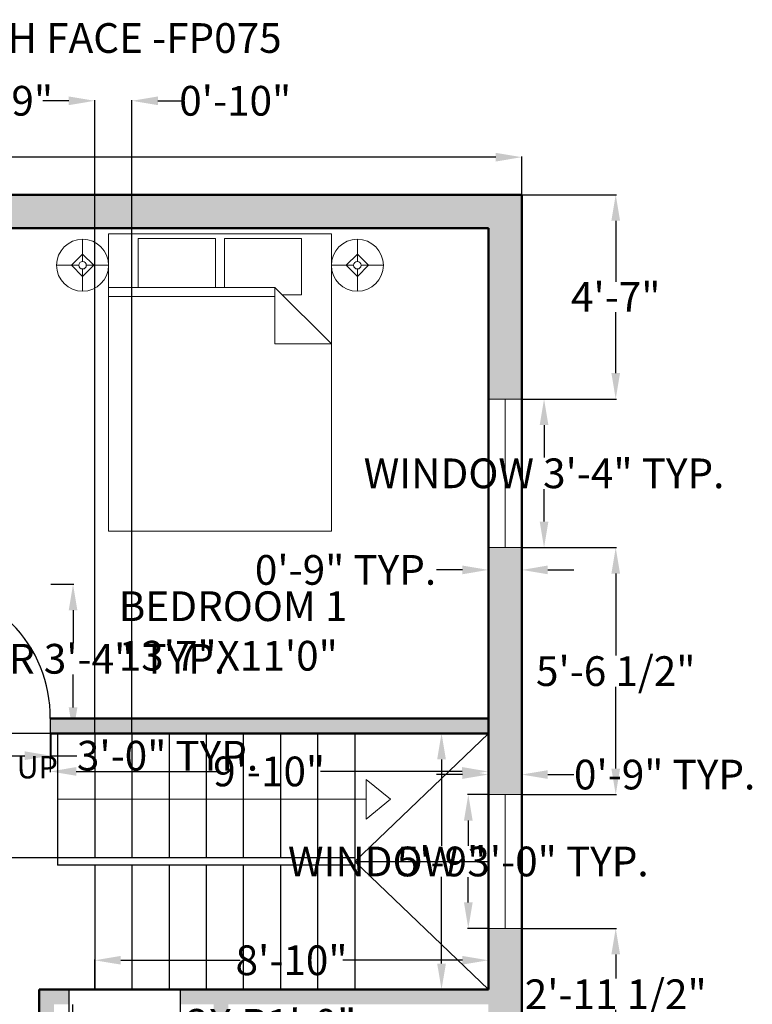
# Model space of a CAD drawing. Units: inches. Extents: x 808573 to 809030, y 884276 to 884799.
# Tile 4 of 4: x 808832 to 809030, y 884534 to 884799. Entities that reach past the tile are written whole.
import ezdxf

# ---------------------------------------------------------------- set-up
doc = ezdxf.new("R2010")
doc.units = ezdxf.units.IN
doc.header["$MEASUREMENT"] = 0
for name, color, linetype, lineweight in [('A-ANNO-DIMS', 2, 'Continuous', 18), ('A-ANNO-SYMB', 7, 'Continuous', 18), ('A-ANNO-TEXT', 7, 'Continuous', 25), ('A-AREA-IDEN', 7, 'Continuous', 25), ('A-DOOR', 3, 'Continuous', 25), ('A-FLOR-STRS', 7, 'Continuous', 25), ('A-FURN', 8, 'Continuous', 18), ('A-GLAZ', 4, 'Continuous', 18), ('A-WALL', 7, 'Continuous', 50)]:
    doc.layers.add(name, color=color, linetype=linetype, lineweight=lineweight)
doc.layers.add('A-WALL-PATT', color=251, linetype='Continuous', lineweight=13, true_color=0x636466)
doc.styles.get("Standard").update_dxf_attribs({"font": 'arial.ttf'})
doc.dimstyles.get("Standard").update_dxf_attribs({"dimtxt": 8, "dimasz": 7, "dimexe": 0.18, "dimexo": 0.0625, "dimgap": 0.09, "dimtad": 0, "dimtih": 1, "dimtoh": 1, "dimdec": 0, "dimzin": 0, "dimdsep": 46, "dimlunit": 3, "dimtxsty": 'Standard', "dimcen": 0.09, "dimadec": 0, "dimazin": 0, "dimtfac": 1, "dimtdec": 0, "dimtofl": 0, "dimtmove": 0, "dimatfit": 3, "dimfxl": 1, "dimtolj": 1, "dimtzin": 0, "dimarcsym": 0})

# ---------------------------------------------------------------- blocks, each defined once
blk = doc.blocks.new('Bed - Queen')
for p, q in [((0, -80.00003), (0, 0)), ((0, 0), (59.99999, 0)), ((59.99999, 0), (59.99999, -80.00003)), ((7.99999, -1.2), (28.79998, -1.2)), ((7.99999, -14.4), (7.99999, -1.2)), ((28.79998, -1.2), (28.79998, -14.4)), ((31.19999, -1.2), (51.99999, -1.2)), ((31.19999, -14.4), (31.19999, -1.2)), ((51.99999, -1.2), (51.99999, -16.4)), ((0, -14.4), (44.8, -14.4)), ((59.99999, -29.6), (44.8, -14.4)), ((44.8, -14.4), (44.8, -29.6)), ((44.8, -16.8), (0, -16.8)), ((51.99999, -16.4), (46.79936, -16.4)), ((44.8, -29.6), (59.99999, -29.6)), ((59.99999, -80.00003), (0, -80.00003))]:
    blk.add_line(p, q)
blk = doc.blocks.new('Lamp - Table')
for p, q in [((0, 7), (0, 1)), ((0, 3), (-3, 0)), ((3, 0), (0, 3)), ((-1, 0), (-7, 0)), ((-3, 0), (0, -3)), ((0, -3), (3, 0)), ((1, 0), (7, 0)), ((0, -1), (0, -7))]:
    blk.add_line(p, q)
for radius in [7, 1]:
    blk.add_circle((0, 0), radius)
blk = doc.blocks.new('*D6')
at = {"layer": 'A-ANNO-DIMS', "color": 0, "lineweight": -2, "transparency": 16777216}
for p, q in [((808619.63, 884751.7), (808619.63, 884761.94)), ((808626.63, 884761.76), (808786.68, 884761.76)), ((808960.63, 884761.76), (808800.58, 884761.76)), ((808967.63, 884751.7), (808967.63, 884761.94))]:
    blk.add_line(p, q, dxfattribs=at)
at = {"layer": 'A-ANNO-DIMS', "color": 0, "transparency": 16777216}
for points in [[(808626.63, 884762.92), (808626.63, 884760.59), (808619.63, 884761.76)], [(808960.63, 884762.92), (808960.63, 884760.59), (808967.63, 884761.76)]]:
    blk.add_solid(points, dxfattribs=at)
at = {"layer": 'Defpoints', "color": 0, "transparency": 16777216}
for p in [(808967.63, 884761.76), (808619.63, 884751.64), (808967.63, 884751.64)]:
    blk.add_point(p, dxfattribs=at)
at = {"layer": 'A-ANNO-DIMS', "color": 0, "transparency": 16777216, "insert": (808793.63, 884761.76), "char_height": 8, "attachment_point": 5}
blk.add_mtext("\\A1;29'", dxfattribs=at)
blk = doc.blocks.new('*D8')
at = {"layer": 'A-ANNO-DIMS', "color": 0, "lineweight": -2, "transparency": 16777216}
for p, q in [((808958.57, 884606.64), (808945.84, 884606.64)), ((808946.02, 884599.64), (808946.02, 884576.31)), ((808946.02, 884544.64), (808946.02, 884567.97)), ((808958.57, 884537.64), (808945.84, 884537.64))]:
    blk.add_line(p, q, dxfattribs=at)
at = {"layer": 'A-ANNO-DIMS', "color": 0, "transparency": 16777216}
for points in [[(808944.85, 884599.64), (808947.19, 884599.64), (808946.02, 884606.64)], [(808944.85, 884544.64), (808947.19, 884544.64), (808946.02, 884537.64)]]:
    blk.add_solid(points, dxfattribs=at)
at = {"layer": 'Defpoints', "color": 0, "transparency": 16777216}
for p in [(808958.63, 884606.64), (808946.02, 884537.64), (808958.63, 884537.64)]:
    blk.add_point(p, dxfattribs=at)
at = {"layer": 'A-ANNO-DIMS', "color": 0, "transparency": 16777216, "insert": (808946.02, 884572.14), "char_height": 8, "attachment_point": 5}
blk.add_mtext('\\A1;5\'-9"', dxfattribs=at)
blk = doc.blocks.new('*D9')
at = {"layer": 'A-ANNO-DIMS', "color": 0, "lineweight": -2, "transparency": 16777216}
for p, q in [((808840.63, 884606.58), (808840.63, 884596.2)), ((808958.57, 884606.58), (808958.57, 884596.2)), ((808847.63, 884596.38), (808885.77, 884596.38)), ((808951.57, 884596.38), (808913.43, 884596.38))]:
    blk.add_line(p, q, dxfattribs=at)
at = {"layer": 'A-ANNO-DIMS', "color": 0, "transparency": 16777216}
for points in [[(808847.63, 884597.55), (808847.63, 884595.22), (808840.63, 884596.38)], [(808951.57, 884597.55), (808951.57, 884595.22), (808958.57, 884596.38)]]:
    blk.add_solid(points, dxfattribs=at)
at = {"layer": 'Defpoints', "color": 0, "transparency": 16777216}
for p in [(808840.63, 884606.64), (808958.57, 884606.64), (808958.57, 884596.38)]:
    blk.add_point(p, dxfattribs=at)
at = {"layer": 'A-ANNO-DIMS', "color": 0, "transparency": 16777216, "insert": (808899.6, 884596.38), "char_height": 8, "attachment_point": 5}
blk.add_mtext('\\A1;9\'-10"', dxfattribs=at)
blk = doc.blocks.new('*D10')
at = {"layer": 'A-ANNO-DIMS', "color": 0, "lineweight": -2, "transparency": 16777216}
for p, q in [((808852.63, 884537.7), (808852.63, 884545.72)), ((808859.63, 884545.54), (808891.79, 884545.54)), ((808951.63, 884545.54), (808919.46, 884545.54)), ((808958.63, 884537.7), (808958.63, 884545.72))]:
    blk.add_line(p, q, dxfattribs=at)
at = {"layer": 'A-ANNO-DIMS', "color": 0, "transparency": 16777216}
for points in [[(808859.63, 884546.71), (808859.63, 884544.38), (808852.63, 884545.54)], [(808951.63, 884546.71), (808951.63, 884544.38), (808958.63, 884545.54)]]:
    blk.add_solid(points, dxfattribs=at)
at = {"layer": 'Defpoints', "color": 0, "transparency": 16777216}
for p in [(808852.63, 884545.54), (808852.63, 884537.64), (808958.63, 884537.64)]:
    blk.add_point(p, dxfattribs=at)
at = {"layer": 'A-ANNO-DIMS', "color": 0, "transparency": 16777216, "insert": (808905.63, 884545.54), "char_height": 8, "attachment_point": 5}
blk.add_mtext('\\A1;8\'-10"', dxfattribs=at)
blk = doc.blocks.new('DOOR-SWING-36IN')
for p, q in [((0, 0), (0, 36)), ((1, 0), (1, 36)), ((0, 0), (0, -4)), ((36, 0), (36, -4))]:
    blk.add_line(p, q)
blk.add_arc((0.5, 0.5), 35.5, 359.1931, 90.8069)
blk = doc.blocks.new('DOOR-SWING-30IN')
for p, q in [((0, 30), (-4, 30)), ((-4, 1), (-34, 1)), ((-4, 0), (-34, 0)), ((0, 0), (-4, 0))]:
    blk.add_line(p, q)
blk.add_arc((-4.5, 0.5), 29.5, 89.029, 180.971)
blk = doc.blocks.new('WIN-40IN')
for p, q in [((0, 0), (9, 0)), ((4.5, 0), (4.5, -40)), ((0, -40), (9, -40))]:
    blk.add_line(p, q)
blk = doc.blocks.new('WIN-36IN')
for p, q in [((0, 0), (-9, 0)), ((-4.5, 0), (-4.5, -36)), ((0, -36), (-9, -36))]:
    blk.add_line(p, q)
blk = doc.blocks.new('*D19')
at = {"layer": 'A-ANNO-DIMS', "color": 0, "lineweight": -2, "transparency": 16777216}
for p, q in [((808840.83, 884646.78), (808846.96, 884646.78)), ((808846.78, 884639.78), (808846.78, 884630.94)), ((808846.78, 884613.64), (808846.78, 884622.48)), ((808840.83, 884606.64), (808846.96, 884606.64))]:
    blk.add_line(p, q, dxfattribs=at)
at = {"layer": 'A-ANNO-DIMS', "color": 0, "transparency": 16777216}
for points in [[(808845.62, 884639.78), (808847.95, 884639.78), (808846.78, 884646.78)], [(808845.62, 884613.64), (808847.95, 884613.64), (808846.78, 884606.64)]]:
    blk.add_solid(points, dxfattribs=at)
at = {"layer": 'Defpoints', "color": 0, "transparency": 16777216}
for p in [(808840.76, 884646.78), (808846.78, 884646.78), (808840.76, 884606.64)]:
    blk.add_point(p, dxfattribs=at)
at = {"layer": 'A-ANNO-DIMS', "color": 0, "transparency": 16777216, "insert": (808846.78, 884626.71), "char_height": 8, "attachment_point": 5}
blk.add_mtext('\\A1;DOOR 3\'-4" TYP.', dxfattribs=at)
blk = doc.blocks.new('*D20')
at = {"layer": 'A-ANNO-DIMS', "color": 0, "lineweight": -2, "transparency": 16777216}
for p, q in [((808804.63, 884606.58), (808804.63, 884600.44)), ((808840.76, 884606.58), (808840.76, 884600.44)), ((808811.63, 884600.62), (808833.76, 884600.62)), ((808840.76, 884600.62), (808847.76, 884600.62))]:
    blk.add_line(p, q, dxfattribs=at)
at = {"layer": 'A-ANNO-DIMS', "color": 0, "transparency": 16777216}
for points in [[(808811.63, 884601.79), (808811.63, 884599.45), (808804.63, 884600.62)], [(808833.76, 884601.79), (808833.76, 884599.45), (808840.76, 884600.62)]]:
    blk.add_solid(points, dxfattribs=at)
at = {"layer": 'Defpoints', "color": 0, "transparency": 16777216}
for p in [(808804.63, 884606.64), (808840.76, 884606.64), (808840.76, 884600.62)]:
    blk.add_point(p, dxfattribs=at)
at = {"layer": 'A-ANNO-DIMS', "color": 0, "transparency": 16777216, "insert": (808872.23, 884600.62), "char_height": 8, "attachment_point": 5}
blk.add_mtext('\\A1;3\'-0" TYP.', dxfattribs=at)
blk = doc.blocks.new('*D23')
at = {"layer": 'A-ANNO-DIMS', "color": 0, "lineweight": -2, "transparency": 16777216}
for p, q in [((808967.69, 884696.64), (808973.81, 884696.64)), ((808973.63, 884689.64), (808973.63, 884680.87)), ((808973.63, 884663.64), (808973.63, 884672.41)), ((808967.69, 884656.64), (808973.81, 884656.64))]:
    blk.add_line(p, q, dxfattribs=at)
at = {"layer": 'A-ANNO-DIMS', "color": 0, "transparency": 16777216}
for points in [[(808972.46, 884689.64), (808974.8, 884689.64), (808973.63, 884696.64)], [(808972.46, 884663.64), (808974.8, 884663.64), (808973.63, 884656.64)]]:
    blk.add_solid(points, dxfattribs=at)
at = {"layer": 'Defpoints', "color": 0, "transparency": 16777216}
for p in [(808967.63, 884696.64), (808967.63, 884656.64), (808973.63, 884656.64)]:
    blk.add_point(p, dxfattribs=at)
at = {"layer": 'A-ANNO-DIMS', "color": 0, "transparency": 16777216, "insert": (808973.63, 884676.64), "char_height": 8, "attachment_point": 5}
blk.add_mtext('\\A1;WINDOW 3\'-4" TYP.', dxfattribs=at)
blk = doc.blocks.new('*D24')
at = {"layer": 'A-ANNO-DIMS', "color": 0, "lineweight": -2, "transparency": 16777216}
for p, q in [((808958.63, 884656.58), (808958.63, 884650.46)), ((808967.63, 884656.58), (808967.63, 884650.46)), ((808951.63, 884650.64), (808944.63, 884650.64)), ((808974.63, 884650.64), (808981.63, 884650.64))]:
    blk.add_line(p, q, dxfattribs=at)
at = {"layer": 'A-ANNO-DIMS', "color": 0, "transparency": 16777216}
for points in [[(808951.63, 884651.81), (808951.63, 884649.47), (808958.63, 884650.64)], [(808974.63, 884651.81), (808974.63, 884649.47), (808967.63, 884650.64)]]:
    blk.add_solid(points, dxfattribs=at)
at = {"layer": 'Defpoints', "color": 0, "transparency": 16777216}
for p in [(808958.63, 884656.64), (808967.63, 884656.64), (808958.63, 884650.64)]:
    blk.add_point(p, dxfattribs=at)
at = {"layer": 'A-ANNO-DIMS', "color": 0, "transparency": 16777216, "insert": (808920.16, 884650.64), "char_height": 8, "attachment_point": 5}
blk.add_mtext('\\A1;0\'-9" TYP.', dxfattribs=at)
blk = doc.blocks.new('*D25')
at = {"layer": 'A-ANNO-DIMS', "color": 0, "lineweight": -2, "transparency": 16777216}
for p, q in [((808958.57, 884590.14), (808953.05, 884590.14)), ((808953.23, 884583.14), (808953.23, 884576.37)), ((808953.23, 884561.14), (808953.23, 884567.91)), ((808958.57, 884554.14), (808953.05, 884554.14))]:
    blk.add_line(p, q, dxfattribs=at)
at = {"layer": 'A-ANNO-DIMS', "color": 0, "transparency": 16777216}
for points in [[(808952.06, 884583.14), (808954.4, 884583.14), (808953.23, 884590.14)], [(808952.06, 884561.14), (808954.4, 884561.14), (808953.23, 884554.14)]]:
    blk.add_solid(points, dxfattribs=at)
at = {"layer": 'Defpoints', "color": 0, "transparency": 16777216}
for p in [(808953.23, 884590.14), (808958.63, 884590.14), (808958.63, 884554.14)]:
    blk.add_point(p, dxfattribs=at)
at = {"layer": 'A-ANNO-DIMS', "color": 0, "transparency": 16777216, "insert": (808953.23, 884572.14), "char_height": 8, "attachment_point": 5}
blk.add_mtext('\\A1;WINDOW 3\'-0" TYP.', dxfattribs=at)
blk = doc.blocks.new('*D26')
at = {"layer": 'A-ANNO-DIMS', "color": 0, "lineweight": -2, "transparency": 16777216}
for p, q in [((808951.63, 884595.54), (808944.63, 884595.54)), ((808958.63, 884590.2), (808958.63, 884595.72)), ((808967.63, 884590.2), (808967.63, 884595.72)), ((808974.63, 884595.54), (808981.63, 884595.54))]:
    blk.add_line(p, q, dxfattribs=at)
at = {"layer": 'A-ANNO-DIMS', "color": 0, "transparency": 16777216}
for points in [[(808951.63, 884596.71), (808951.63, 884594.37), (808958.63, 884595.54)], [(808974.63, 884596.71), (808974.63, 884594.37), (808967.63, 884595.54)]]:
    blk.add_solid(points, dxfattribs=at)
at = {"layer": 'Defpoints', "color": 0, "transparency": 16777216}
for p in [(808967.63, 884595.54), (808958.63, 884590.14), (808967.63, 884590.14)]:
    blk.add_point(p, dxfattribs=at)
at = {"layer": 'A-ANNO-DIMS', "color": 0, "transparency": 16777216, "insert": (809006.1, 884595.54), "char_height": 8, "attachment_point": 5}
blk.add_mtext('\\A1;0\'-9" TYP.', dxfattribs=at)
blk = doc.blocks.new('*D36')
at = {"layer": 'A-ANNO-DIMS', "color": 0, "lineweight": -2, "transparency": 16777216}
for p, q in [((808967.69, 884751.64), (808993.11, 884751.64)), ((808992.93, 884744.64), (808992.93, 884728.23)), ((808992.93, 884703.64), (808992.93, 884720.05)), ((808967.69, 884696.64), (808993.11, 884696.64))]:
    blk.add_line(p, q, dxfattribs=at)
at = {"layer": 'A-ANNO-DIMS', "color": 0, "transparency": 16777216}
for points in [[(808991.76, 884744.64), (808994.1, 884744.64), (808992.93, 884751.64)], [(808991.76, 884703.64), (808994.1, 884703.64), (808992.93, 884696.64)]]:
    blk.add_solid(points, dxfattribs=at)
at = {"layer": 'Defpoints', "color": 0, "transparency": 16777216}
for p in [(808967.63, 884751.64), (808967.63, 884696.64), (808992.93, 884696.64)]:
    blk.add_point(p, dxfattribs=at)
at = {"layer": 'A-ANNO-DIMS', "color": 0, "transparency": 16777216, "insert": (808992.93, 884724.14), "char_height": 8, "attachment_point": 5}
blk.add_mtext('\\A1;4\'-7"', dxfattribs=at)
blk = doc.blocks.new('*D37')
at = {"layer": 'A-ANNO-DIMS', "color": 0, "lineweight": -2, "transparency": 16777216}
for p, q in [((808967.69, 884656.64), (808993.11, 884656.64)), ((808992.93, 884649.64), (808992.93, 884627.62)), ((808992.93, 884597.14), (808992.93, 884619.16)), ((808967.69, 884590.14), (808993.11, 884590.14))]:
    blk.add_line(p, q, dxfattribs=at)
at = {"layer": 'A-ANNO-DIMS', "color": 0, "transparency": 16777216}
for points in [[(808991.76, 884649.64), (808994.1, 884649.64), (808992.93, 884656.64)], [(808991.76, 884597.14), (808994.1, 884597.14), (808992.93, 884590.14)]]:
    blk.add_solid(points, dxfattribs=at)
at = {"layer": 'Defpoints', "color": 0, "transparency": 16777216}
for p in [(808967.63, 884656.64), (808967.63, 884590.14), (808992.93, 884590.14)]:
    blk.add_point(p, dxfattribs=at)
at = {"layer": 'A-ANNO-DIMS', "color": 0, "transparency": 16777216, "insert": (808992.93, 884623.39), "char_height": 8, "attachment_point": 5}
blk.add_mtext('\\A1;5\'-6 1/2"', dxfattribs=at)
blk = doc.blocks.new('*D39')
at = {"layer": 'A-ANNO-DIMS', "color": 0, "lineweight": -2, "transparency": 16777216}
for p, q in [((808967.69, 884554.14), (808993.11, 884554.14)), ((808992.93, 884547.14), (808992.93, 884540.62)), ((808992.93, 884525.64), (808992.93, 884532.16)), ((808967.69, 884518.64), (808993.11, 884518.64))]:
    blk.add_line(p, q, dxfattribs=at)
at = {"layer": 'A-ANNO-DIMS', "color": 0, "transparency": 16777216}
for points in [[(808991.76, 884547.14), (808994.1, 884547.14), (808992.93, 884554.14)], [(808991.76, 884525.64), (808994.1, 884525.64), (808992.93, 884518.64)]]:
    blk.add_solid(points, dxfattribs=at)
at = {"layer": 'Defpoints', "color": 0, "transparency": 16777216}
for p in [(808967.63, 884554.14), (808992.93, 884554.14), (808967.63, 884518.64)]:
    blk.add_point(p, dxfattribs=at)
at = {"layer": 'A-ANNO-DIMS', "color": 0, "transparency": 16777216, "insert": (808992.93, 884536.39), "char_height": 8, "attachment_point": 5}
blk.add_mtext('\\A1;2\'-11 1/2"', dxfattribs=at)
blk = doc.blocks.new('*D47')
at = {"layer": 'A-ANNO-DIMS', "color": 0, "lineweight": -2, "transparency": 16777216}
for p, q in [((808845.63, 884776.94), (808838.63, 884776.94)), ((808852.63, 884606.7), (808852.63, 884777.12)), ((808862.63, 884606.7), (808862.63, 884777.12)), ((808869.63, 884776.94), (808876.63, 884776.94))]:
    blk.add_line(p, q, dxfattribs=at)
at = {"layer": 'A-ANNO-DIMS', "color": 0, "transparency": 16777216}
for points in [[(808845.63, 884778.11), (808845.63, 884775.77), (808852.63, 884776.94)], [(808869.63, 884778.11), (808869.63, 884775.77), (808862.63, 884776.94)]]:
    blk.add_solid(points, dxfattribs=at)
at = {"layer": 'Defpoints', "color": 0, "transparency": 16777216}
for p in [(808862.63, 884776.94), (808852.63, 884606.64), (808862.63, 884606.64)]:
    blk.add_point(p, dxfattribs=at)
at = {"layer": 'A-ANNO-DIMS', "color": 0, "transparency": 16777216, "insert": (808890.46, 884776.94), "char_height": 8, "attachment_point": 5}
blk.add_mtext('\\A1;0\'-10"', dxfattribs=at)
blk = doc.blocks.new('*D49')
at = {"layer": 'A-ANNO-DIMS', "color": 0, "lineweight": -2, "transparency": 16777216}
for p, q in [((808788.63, 884776.94), (808781.63, 884776.94)), ((808795.63, 884610.7), (808795.63, 884777.12)), ((808804.63, 884610.7), (808804.63, 884777.12)), ((808811.63, 884776.94), (808818.63, 884776.94))]:
    blk.add_line(p, q, dxfattribs=at)
at = {"layer": 'A-ANNO-DIMS', "color": 0, "transparency": 16777216}
for points in [[(808788.63, 884778.11), (808788.63, 884775.77), (808795.63, 884776.94)], [(808811.63, 884778.11), (808811.63, 884775.77), (808804.63, 884776.94)]]:
    blk.add_solid(points, dxfattribs=at)
at = {"layer": 'Defpoints', "color": 0, "transparency": 16777216}
for p in [(808804.63, 884776.94), (808795.63, 884610.64), (808804.63, 884610.64)]:
    blk.add_point(p, dxfattribs=at)
at = {"layer": 'A-ANNO-DIMS', "color": 0, "transparency": 16777216, "insert": (808829.35, 884776.94), "char_height": 8, "attachment_point": 5}
blk.add_mtext('\\A1;0\'-9"', dxfattribs=at)
blk = doc.blocks.new('*D52')
at = {"layer": 'A-ANNO-DIMS', "color": 0, "lineweight": -2, "transparency": 16777216}
for p, q in [((808842.57, 884606.64), (808594.15, 884606.64)), ((808594.33, 884599.64), (808594.33, 884594.12)), ((808594.33, 884580.14), (808594.33, 884585.66)), ((808842.57, 884573.14), (808594.15, 884573.14))]:
    blk.add_line(p, q, dxfattribs=at)
at = {"layer": 'A-ANNO-DIMS', "color": 0, "transparency": 16777216}
for points in [[(808593.16, 884599.64), (808595.5, 884599.64), (808594.33, 884606.64)], [(808593.16, 884580.14), (808595.5, 884580.14), (808594.33, 884573.14)]]:
    blk.add_solid(points, dxfattribs=at)
at = {"layer": 'Defpoints', "color": 0, "transparency": 16777216}
for p in [(808842.63, 884606.64), (808594.33, 884573.14), (808842.63, 884573.14)]:
    blk.add_point(p, dxfattribs=at)
at = {"layer": 'A-ANNO-DIMS', "color": 0, "transparency": 16777216, "insert": (808594.33, 884589.89), "char_height": 8, "attachment_point": 5}
blk.add_mtext('\\A1;2\'-9 1/2"', dxfattribs=at)
blk = doc.blocks.new('*D58')
at = {"layer": 'A-ANNO-DIMS', "color": 0, "lineweight": -2, "transparency": 16777216}
for p, q in [((808923.4, 884528.43), (808930.4, 884528.43)), ((808930.4, 884528.43), (808932.18, 884521.66)), ((808936.96, 884503.12), (808937.14, 884503.12)), ((808937.05, 884503.03), (808937.05, 884503.21))]:
    blk.add_line(p, q, dxfattribs=at)
at = {"layer": 'A-ANNO-DIMS', "color": 0, "transparency": 16777216}
blk.add_solid([(808933.31, 884521.96), (808931.05, 884521.36), (808933.96, 884514.89)], dxfattribs=at)
at = {"layer": 'Defpoints', "color": 0, "transparency": 16777216}
for p in [(808933.96, 884514.89), (808937.05, 884503.12)]:
    blk.add_point(p, dxfattribs=at)
at = {"layer": 'A-ANNO-DIMS', "color": 0, "transparency": 16777216, "insert": (808900.18, 884528.43), "char_height": 8, "attachment_point": 5}
blk.add_mtext('\\A1;2X R1\'-0"', dxfattribs=at)

msp = doc.modelspace()

# ---------------------------------------------------------------- hatches: boundary and pattern name
at = {"layer": 'A-WALL-PATT'}
h = msp.add_hatch(color=256, dxfattribs=at)
h.dxf.hatch_style = 1
h.paths.add_polyline_path([(808967.63, 884751.64), (808619.63, 884751.64), (808619.63, 884696.64), (808628.63, 884696.64), (808628.63, 884742.64), (808791.63, 884742.64), (808958.63, 884742.64), (808958.63, 884696.64), (808967.63, 884696.64)])
h.paths.add_polyline_path([(808967.63, 884656.64), (808958.63, 884656.64), (808958.63, 884610.64), (808958.63, 884590.14), (808967.63, 884590.14)])
h.paths.add_polyline_path([(808967.63, 884494.64), (808958.63, 884494.64), (808958.63, 884479.64), (808958.63, 884340.64), (808901.23, 884340.64), (808901.23, 884331.64), (808967.63, 884331.64)])
h.paths.add_polyline_path([(808967.63, 884554.14), (808958.63, 884554.14), (808958.63, 884537.64), (808875.63, 884537.64), (808875.63, 884533.64), (808884.63, 884533.64), (808884.63, 884479.64), (808841.63, 884479.64), (808841.63, 884533.64), (808845.63, 884533.64), (808845.63, 884537.64), (808837.63, 884537.64), (808837.63, 884479.64), (808837.63, 884475.64), (808958.63, 884475.64), (808958.63, 884479.64), (808888.63, 884479.64), (808888.63, 884533.64), (808958.63, 884533.64), (808958.63, 884518.64), (808967.63, 884518.64)])
h.paths.add_polyline_path([(808858.03, 884340.64), (808800.63, 884340.64), (808800.63, 884365.64), (808791.63, 884365.64), (808791.63, 884331.64), (808858.03, 884331.64)])
h.paths.add_polyline_path([(808800.63, 884475.64), (808801.63, 884475.64), (808801.63, 884479.64), (808791.63, 884479.64), (808791.63, 884430.64), (808791.63, 884405.64), (808800.63, 884405.64)])
h.paths.add_polyline_path([(808740.63, 884434.64), (808704.63, 884434.64), (808704.63, 884438.64), (808700.63, 884438.64), (808700.63, 884434.64), (808628.63, 884434.64), (808628.63, 884443.64), (808619.63, 884443.64), (808619.63, 884430.64), (808740.63, 884430.64)])
h.paths.add_polyline_path([(808628.63, 884528.64), (808619.63, 884528.64), (808619.63, 884473.64), (808628.63, 884473.64), (808628.63, 884482.64)])
h.paths.add_polyline_path([(808628.63, 884606.64), (808628.63, 884656.64), (808619.63, 884656.64), (808619.63, 884564.64), (808628.63, 884564.64)])
h.paths.add_polyline_path([(808704.63, 884482.64), (808704.63, 884495.59), (808700.63, 884495.59), (808700.63, 884486.64), (808628.63, 884486.64), (808628.63, 884482.64), (808700.63, 884482.64), (808700.63, 884468.64), (808704.63, 884468.64)])
h.paths.add_polyline_path([(808704.63, 884606.64), (808700.63, 884606.64), (808700.63, 884531.59), (808704.63, 884531.59)])
h.paths.add_polyline_path([(808746.63, 884610.64), (808628.63, 884610.64), (808628.63, 884606.64), (808746.63, 884606.64)])
h.paths.add_polyline_path([(808804.63, 884610.64), (808795.63, 884610.64), (808795.63, 884742.64), (808791.63, 884742.64), (808791.63, 884610.64), (808782.63, 884610.64), (808782.63, 884606.64), (808804.63, 884606.64)])
h.paths.add_polyline_path([(808958.63, 884610.64), (808840.63, 884610.64), (808840.63, 884606.64), (808958.63, 884606.64)])

# ---------------------------------------------------------------- linework, layer by layer
at = {"layer": 'A-ANNO-SYMB'}
for p, q in [((808925.73, 884588.89), (808925.73, 884594.22)), ((808925.73, 884594.22), (808932.24, 884588.89)), ((808842.63, 884588.89), (808922.63, 884588.89)), ((808922.63, 884588.89), (808925.73, 884588.89)), ((808925.73, 884588.89), (808925.73, 884583.56)), ((808925.73, 884583.56), (808932.24, 884588.89))]:
    msp.add_line(p, q, dxfattribs=at)
at = {"layer": 'A-FLOR-STRS'}
for p, q in [((808842.63, 884606.64), (808842.63, 884571.14)), ((808852.63, 884606.64), (808852.63, 884573.14)), ((808862.63, 884606.64), (808862.63, 884573.14)), ((808872.63, 884606.64), (808872.63, 884573.14)), ((808882.63, 884606.64), (808882.63, 884573.14)), ((808892.63, 884606.64), (808892.63, 884573.14)), ((808902.63, 884606.64), (808902.63, 884573.14)), ((808912.63, 884606.64), (808912.63, 884573.14)), ((808922.63, 884606.64), (808922.63, 884537.64)), ((808922.63, 884572.14), (808958.63, 884606.64)), ((808922.63, 884573.14), (808842.63, 884573.14)), ((808922.63, 884571.14), (808842.63, 884571.14)), ((808852.63, 884571.14), (808852.63, 884537.64)), ((808862.63, 884571.14), (808862.63, 884537.64)), ((808872.63, 884571.14), (808872.63, 884537.64)), ((808882.63, 884571.14), (808882.63, 884537.64)), ((808892.63, 884571.14), (808892.63, 884537.64)), ((808902.63, 884571.14), (808902.63, 884537.64)), ((808912.63, 884571.14), (808912.63, 884537.64)), ((808922.63, 884572.14), (808958.63, 884572.14)), ((808922.63, 884572.14), (808958.63, 884537.64))]:
    msp.add_line(p, q, dxfattribs=at)
at = {"layer": 'A-WALL'}
for p, q in [((808619.63, 884751.64), (808967.63, 884751.64)), ((808967.63, 884751.64), (808967.63, 884331.64)), ((808791.63, 884742.64), (808958.63, 884742.64)), ((808958.63, 884742.64), (808958.63, 884610.64)), ((808840.63, 884610.64), (808958.63, 884610.64)), ((808958.63, 884610.64), (808958.63, 884537.64)), ((808840.63, 884606.64), (808958.63, 884606.64)), ((808958.63, 884537.64), (808837.63, 884537.64)), ((808837.63, 884537.64), (808837.63, 884479.64))]:
    msp.add_line(p, q, dxfattribs=at)

# ---------------------------------------------------------------- block references
at = {"layer": 'A-DOOR'}
msp.add_blockref('DOOR-SWING-36IN', (808804.63, 884610.64), dxfattribs=at)
at = {"layer": 'A-DOOR', "extrusion": (0, 0, -1), "zscale": -1, "rotation": 89.99999999926234}
msp.add_blockref('DOOR-SWING-30IN', (-808845.63, 884537.64), dxfattribs=at)
at = {"layer": 'A-FURN'}
for name, p in [('Lamp - Table', (808849.35, 884732.66)), ('Bed - Queen', (808856.35, 884741.09))]:
    msp.add_blockref(name, p, dxfattribs=at)
at = {"layer": 'A-FURN', "xscale": -1}
msp.add_blockref('Lamp - Table', (808923.35, 884732.66), dxfattribs=at)
at = {"layer": 'A-GLAZ', "rotation": 180}
msp.add_blockref('WIN-40IN', (808967.63, 884656.64), dxfattribs=at)
at = {"layer": 'A-GLAZ'}
msp.add_blockref('WIN-36IN', (808967.63, 884590.14), dxfattribs=at)

# ---------------------------------------------------------------- texts
at = {"layer": 'A-ANNO-TEXT', "attachment_point": 1}
for s, width, heights, insert, char_height in [('{\\fArial|b1|i0|c0|p34;29X35 (1015 SQFT) HOUSE PLAN - NORTH FACE -FP075}', 304.7381, [0.175], (808627.8, 884797.84), 8), (' UP', 9.0759, [0], (808831.61, 884600.51), 6)]:
    msp.add_mtext_dynamic_manual_height_columns(s, width=width, gutter_width=1, heights=heights, dxfattribs=dict(at, insert=insert, char_height=char_height))
at = {"layer": 'A-AREA-IDEN', "insert": (808859.08, 884644.87), "char_height": 8, "attachment_point": 1}
msp.add_mtext_dynamic_manual_height_columns('BEDROOM 1\\P13\'7"X11\'0"', width=94.1107, gutter_width=1, heights=[0], dxfattribs=at)

# ---------------------------------------------------------------- dimensions: what is measured, and where the dimension line sits
at = {"layer": 'A-ANNO-DIMS'}
for base, p1, p2, override, picture, middle in [((808804.63, 884776.94), (808795.63, 884610.64), (808804.63, 884610.64), {"dimdec": 1, "dimlfac": 1, "dimrnd": 0, "dimzin": 1, "dimdsep": 46, "dimlunit": 4, "dimfrac": 2}, '*D49', (808829.35, 884776.94)), ((808862.63, 884776.94), (808852.63, 884606.64), (808862.63, 884606.64), {"dimdec": 1, "dimlfac": 1, "dimrnd": 0, "dimzin": 1, "dimdsep": 46, "dimlunit": 4, "dimfrac": 2}, '*D47', (808890.46, 884776.94)), ((808967.63, 884761.76), (808619.63, 884751.64), (808967.63, 884751.64), {"dimclrd": 0, "dimclre": 0, "dimclrt": 0}, '*D6', (808793.63, 884761.76)), ((808958.57, 884596.38), (808840.63, 884606.64), (808958.57, 884606.64), {"dimclrd": 0, "dimclre": 0, "dimclrt": 0}, '*D9', (808899.6, 884596.38)), ((808852.63, 884545.54), (808958.63, 884537.64), (808852.63, 884537.64), {"dimclrd": 0, "dimclre": 0, "dimclrt": 0}, '*D10', (808905.63, 884545.54))]:
    dim = msp.add_linear_dim(base=base, p1=p1, p2=p2, dimstyle='Standard', override=override, dxfattribs=at)
    dim.commit()
    dim.dimension.update_dxf_attribs({"geometry": picture, "text_midpoint": middle})
for base, p1, p2, override, picture, middle in [((808992.93, 884696.64), (808967.63, 884751.64), (808967.63, 884696.64), {"dimdec": 1, "dimlfac": 1, "dimrnd": 0, "dimzin": 1, "dimdsep": 46, "dimlunit": 4, "dimfrac": 2}, '*D36', (808992.93, 884724.14)), ((808992.93, 884590.14), (808967.63, 884656.64), (808967.63, 884590.14), {"dimdec": 1, "dimlfac": 1, "dimrnd": 0, "dimzin": 1, "dimdsep": 46, "dimlunit": 4, "dimfrac": 2}, '*D37', (808992.93, 884623.39)), ((808594.33, 884573.14), (808842.63, 884606.64), (808842.63, 884573.14), {"dimdec": 1, "dimlfac": 1, "dimrnd": 0, "dimzin": 1, "dimdsep": 46, "dimlunit": 4, "dimfrac": 2}, '*D52', (808594.33, 884589.89)), ((808946.02, 884537.64), (808958.63, 884606.64), (808958.63, 884537.64), {"dimclrd": 0, "dimclre": 0, "dimclrt": 0}, '*D8', (808946.02, 884572.14)), ((808992.93, 884554.14), (808967.63, 884518.64), (808967.63, 884554.14), {"dimdec": 1, "dimlfac": 1, "dimrnd": 0, "dimzin": 1, "dimdsep": 46, "dimlunit": 4, "dimfrac": 2}, '*D39', (808992.93, 884536.39))]:
    dim = msp.add_linear_dim(base=base, p1=p1, p2=p2, angle=90, dimstyle='Standard', override=override, dxfattribs=at)
    dim.commit()
    dim.dimension.update_dxf_attribs({"geometry": picture, "text_midpoint": middle})
for base, p1, p2, angle, text, picture, middle in [((808973.63, 884656.64), (808967.63, 884696.64), (808967.63, 884656.64), 270, 'WINDOW <> TYP.', '*D23', (808973.63, 884676.64)), ((808958.63, 884650.64), (808967.63, 884656.64), (808958.63, 884656.64), 180, '<> TYP.', '*D24', (808920.16, 884650.64)), ((808846.78, 884646.78), (808840.76, 884606.64), (808840.76, 884646.78), 90, 'DOOR <> TYP.', '*D19', (808846.78, 884626.71)), ((808953.23, 884590.14), (808958.63, 884554.14), (808958.63, 884590.14), 90, 'WINDOW <> TYP.', '*D25', (808953.23, 884572.14))]:
    dim = msp.add_linear_dim(base=base, p1=p1, p2=p2, angle=angle, text=text, dimstyle='Standard', override={"dimdec": 1, "dimlfac": 1, "dimrnd": 0, "dimzin": 1, "dimdsep": 46, "dimlunit": 4, "dimfrac": 2}, dxfattribs=at)
    dim.commit()
    dim.dimension.update_dxf_attribs({"geometry": picture, "text_midpoint": middle})
for base, p1, p2, picture, middle in [((808840.76, 884600.62), (808804.63, 884606.64), (808840.76, 884606.64), '*D20', (808872.23, 884600.62)), ((808967.63, 884595.54), (808958.63, 884590.14), (808967.63, 884590.14), '*D26', (809006.1, 884595.54))]:
    dim = msp.add_linear_dim(base=base, p1=p1, p2=p2, text='<> TYP.', dimstyle='Standard', override={"dimdec": 1, "dimlfac": 1, "dimrnd": 0, "dimzin": 1, "dimdsep": 46, "dimlunit": 4, "dimfrac": 2}, dxfattribs=at)
    dim.commit()
    dim.dimension.update_dxf_attribs({"geometry": picture, "text_midpoint": middle})
dim = msp.add_radius_dim(center=(808937.05, 884503.12), mpoint=(808933.96, 884514.89), text='2X <>', dimstyle='Standard', override={"dimdec": 1, "dimlfac": 1, "dimrnd": 0, "dimzin": 1, "dimdsep": 46, "dimlunit": 4, "dimfrac": 2}, dxfattribs=at)
dim.commit()
dim.dimension.update_dxf_attribs({"geometry": '*D58', "text_midpoint": (808900.18, 884528.43)})

doc.saveas('drawing.dxf')
